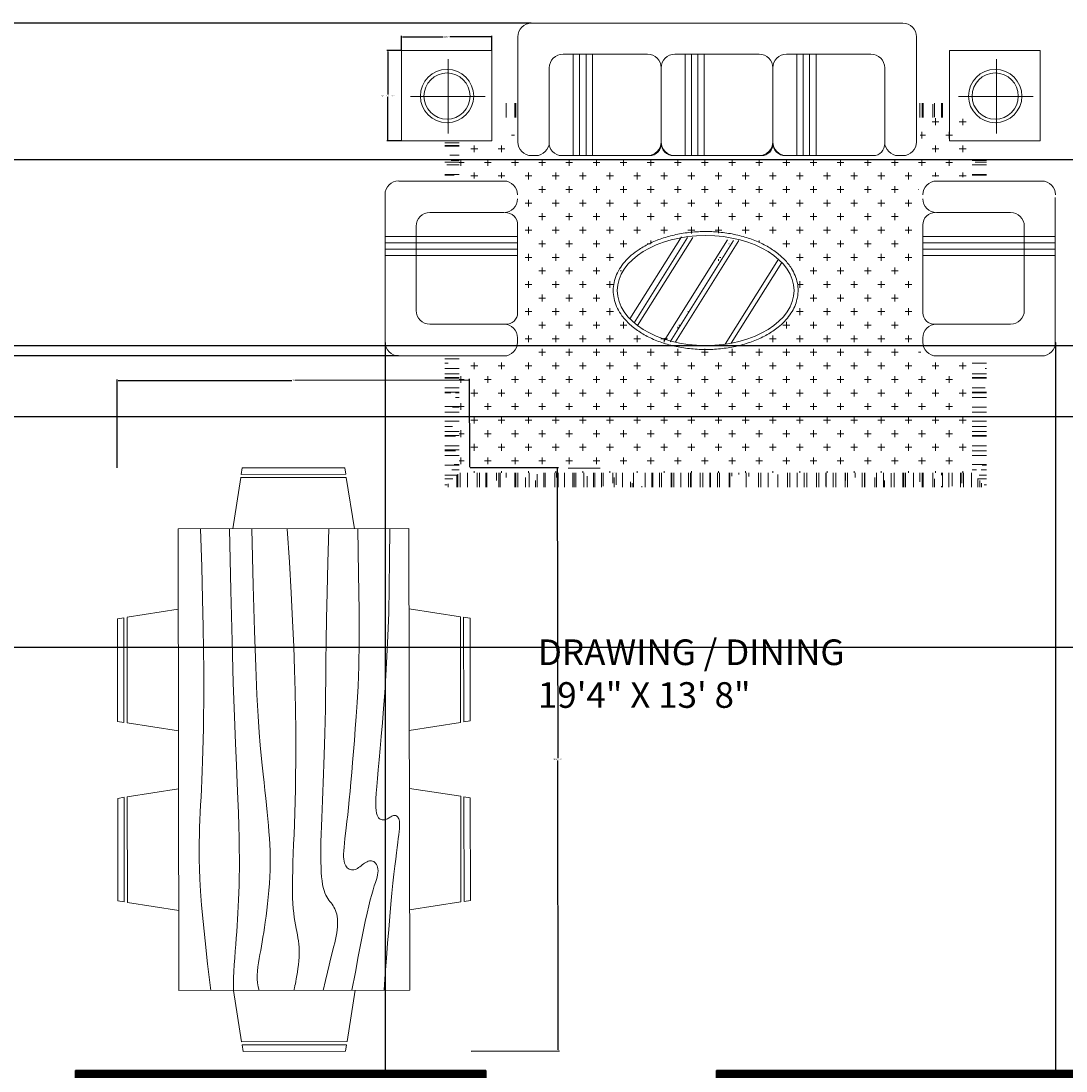
# Model space of a CAD drawing. Units: inches. Extents: x -24 to 516, y -23 to 640.
# Tile 3 of 5: x 139 to 302, y 288 to 452. Entities that reach past the tile are written whole.
import ezdxf

# ---------------------------------------------------------------- set-up
doc = ezdxf.new("R2010")
doc.units = ezdxf.units.IN
doc.header["$MEASUREMENT"] = 0
for name, color, linetype, lineweight in [('A-ANNO-DIMS', 2, 'Continuous', 18), ('A-AREA-IDEN', 7, 'Continuous', 18), ('A-FURN-PATT', 8, 'Continuous', 13), ('A-WALL', 7, 'Continuous', 35), ('furniture', 220, 'Continuous', 18)]:
    doc.layers.add(name, color=color, linetype=linetype, lineweight=lineweight)
doc.layers.add('A-WALL-PATT', color=198, linetype='Continuous', lineweight=13, true_color=0x2e0f2e)
doc.styles.get("Standard").update_dxf_attribs({"font": 'arial.ttf'})
doc.dimstyles.get("Standard").update_dxf_attribs({"dimtxt": 0.18, "dimasz": 0.18, "dimexe": 0.18, "dimexo": 0.0625, "dimgap": 0.09, "dimtad": 0, "dimtih": 1, "dimtoh": 1, "dimdec": 4, "dimzin": 0, "dimdsep": 46, "dimtxsty": 'Standard', "dimcen": 0.09, "dimadec": 0, "dimazin": 0, "dimtfac": 1, "dimtdec": 4, "dimtofl": 0, "dimtmove": 0, "dimatfit": 3, "dimfxl": 1, "dimtolj": 1, "dimtzin": 0, "dimarcsym": 0})

# ---------------------------------------------------------------- blocks, each defined once
blk = doc.blocks.new('Dining Set - 36 x 72 in.')
for p, q in [((-22, 27.5), (-22.1562, 26.50042)), ((-5.8416, 26.5), (-22.1534, 26.5)), ((-22, 27.5), (-6, 27.5)), ((-5.8437, 26.49966), (-6, 27.5)), ((6, 27.5), (5.8438, 26.50042)), ((22.1584, 26.5), (5.8466, 26.5)), ((6, 27.5), (22, 27.5)), ((22.1563, 26.49966), (22, 27.5)), ((-22.2343, 26.00059), (-23.4847, 17.99762)), ((-22.2304, 26), (-5.7608, 26)), ((-4.5152, 17.99762), (-5.7655, 25.99926)), ((5.7657, 26.00059), (4.5153, 17.99762)), ((5.7696, 26), (22.2392, 26)), ((23.4848, 17.99762), (22.2345, 25.99926)), ((36, 18), (-36, 18)), ((-36, 18), (-36, -18)), ((36, -18), (36, 18)), ((-44.0006, 8.23428), (-35.9976, 9.48474)), ((-44, 8.23041), (-44, -8.23915)), ((44.0006, 8.23428), (35.9976, 9.48474)), ((44, 8.23041), (44, -8.23915)), ((-45.5, 8), (-44.5004, 8.15617)), ((-45.5, 8), (-45.5, -8)), ((-44.5, -8.15843), (-44.5, 8.15338)), ((44.5, -8.15843), (44.5, 8.15338)), ((45.5, 8), (44.5005, 8.15617)), ((45.5, 8), (45.5, -8)), ((-44.4997, -8.15631), (-45.5, -8)), ((44.4997, -8.15631), (45.5, -8)), ((-35.9976, -9.48476), (-43.9993, -8.2345)), ((35.9976, -9.48476), (43.9993, -8.2345)), ((-36, -18), (36, -18)), ((-22.2343, -26.0006), (-23.4847, -17.99762)), ((-4.5152, -17.99762), (-5.7655, -25.99928)), ((5.7657, -26.0006), (4.5153, -17.99762)), ((23.4848, -17.99762), (22.2345, -25.99928)), ((-22.2304, -26), (-5.7608, -26)), ((5.7696, -26), (22.2392, -26)), ((-22, -27.5), (-22.1562, -26.50044)), ((-5.8416, -26.5), (-22.1534, -26.5)), ((-22, -27.5), (-6, -27.5)), ((-5.8437, -26.49967), (-6, -27.5)), ((6, -27.5), (5.8438, -26.50044)), ((22.1584, -26.5), (5.8466, -26.5)), ((6, -27.5), (22, -27.5)), ((22.1563, -26.49967), (22, -27.5))]:
    blk.add_line(p, q)
for points in [[(-36, 15), (-31.1772, 14.97754), (-26.8079, 14.91406), (-22.8538, 14.81543), (-19.276, 14.6875), (-16.0362, 14.53613), (-13.0957, 14.36718), (-10.4159, 14.18652), (-7.9583, 14), (-5.6904, 13.81315), (-3.6035, 13.63021), (-1.6954, 13.45508), (0.0365, 13.29166), (1.5945, 13.14388), (2.9811, 13.01562), (4.1988, 12.9108), (5.25, 12.83333), (6.1393, 12.78613), (6.8802, 12.76823), (7.4883, 12.77767), (7.9792, 12.8125), (8.3685, 12.87077), (8.6719, 12.95052), (8.9049, 13.0498), (9.0833, 13.16666), (9.2205, 13.29899), (9.3216, 13.44401), (9.3895, 13.59879), (9.4271, 13.76041), (9.4373, 13.92594), (9.4232, 14.09245), (9.3875, 14.257), (9.3333, 14.41666), (9.2638, 14.56917), (9.1836, 14.71484), (9.0975, 14.85465), (9.0104, 14.98958), (8.9272, 15.1206), (8.8529, 15.2487), (8.7922, 15.37483), (8.75, 15.5), (8.7305, 15.62467), (8.7344, 15.74739), (8.7617, 15.86621), (8.8125, 15.97916), (8.8867, 16.08431), (8.9844, 16.17968), (9.1055, 16.26334), (9.25, 16.33333), (9.4189, 16.38802), (9.6172, 16.42708), (9.8506, 16.45052), (10.125, 16.45833), (10.4463, 16.45052), (10.8203, 16.42708), (11.2529, 16.38802), (11.75, 16.33333), (12.3184, 16.26318), (12.9694, 16.17838), (13.7151, 16.07991), (14.5677, 15.96875), (15.5395, 15.84586), (16.6426, 15.71224), (17.8893, 15.56884), (19.2917, 15.41666), (20.859, 15.25667), (22.5879, 15.08984), (24.4721, 14.91715), (26.5052, 14.73958), (28.6809, 14.5581), (30.9929, 14.3737), (33.4347, 14.18733), (36, 14)], [(-36, 10), (-28.9766, 10.14274), (-23.1725, 10.20442), (-18.4241, 10.19775), (-14.5677, 10.13541), (-11.4399, 10.03011), (-8.877, 9.89453), (-6.7154, 9.74137), (-4.7917, 9.58333), (-2.9698, 9.43082), (-1.2246, 9.28515), (0.4415, 9.14534), (2.026, 9.01041), (3.5266, 8.87939), (4.9408, 8.7513), (6.266, 8.62516), (7.5, 8.5), (8.6411, 8.37549), (9.6914, 8.2539), (10.6538, 8.13818), (11.5312, 8.03125), (12.3267, 7.93603), (13.043, 7.85547), (13.6831, 7.79248), (14.25, 7.75), (14.7471, 7.7303), (15.1797, 7.73307), (15.5537, 7.75732), (15.875, 7.80208), (16.1494, 7.86637), (16.3828, 7.94922), (16.5811, 8.04964), (16.75, 8.16666), (16.8944, 8.29915), (17.0143, 8.44531), (17.1089, 8.60319), (17.1771, 8.77083), (17.218, 8.94629), (17.2305, 9.1276), (17.2137, 9.31282), (17.1667, 9.5), (17.0895, 9.6875), (16.987, 9.875), (16.8649, 10.0625), (16.7292, 10.25), (16.5856, 10.4375), (16.4401, 10.625), (16.2985, 10.8125), (16.1667, 11), (16.05, 11.18733), (15.9518, 11.3737), (15.8752, 11.5581), (15.8229, 11.73958), (15.798, 11.91715), (15.8034, 12.08984), (15.842, 12.25667), (15.9167, 12.41666), (16.0295, 12.56836), (16.1784, 12.70833), (16.3605, 12.83268), (16.5729, 12.9375), (16.8127, 13.01888), (17.0768, 13.07291), (17.3625, 13.0957), (17.6667, 13.08333), (17.9894, 13.03312), (18.3418, 12.94726), (18.7382, 12.82918), (19.1927, 12.68229), (19.7195, 12.51001), (20.3327, 12.31575), (21.0465, 12.10294), (21.875, 11.875), (22.8357, 11.63354), (23.959, 11.37304), (25.2786, 11.08618), (26.8282, 10.76562), (28.6414, 10.40405), (30.752, 9.99414), (33.1936, 9.52856), (36, 9)], [(-36, 5.5), (-30.7157, 5.3348), (-26.069, 5.20963), (-21.9946, 5.11767), (-18.4271, 5.05208), (-15.3009, 5.00602), (-12.5508, 4.97265), (-10.1112, 4.94515), (-7.9167, 4.91666), (-5.909, 4.88167), (-4.0586, 4.83984), (-2.3429, 4.79215), (-0.7396, 4.73958), (0.7739, 4.6831), (2.22, 4.6237), (3.6213, 4.56233), (5, 4.5), (6.373, 4.43782), (7.7344, 4.3776), (9.0723, 4.32129), (10.375, 4.27083), (11.6309, 4.22819), (12.8281, 4.19531), (13.9551, 4.17415), (15, 4.16666), (15.954, 4.17448), (16.819, 4.19791), (17.6001, 4.23698), (18.3021, 4.29166), (18.9299, 4.36198), (19.4883, 4.44791), (19.9823, 4.54948), (20.4167, 4.66666), (20.7969, 4.79899), (21.1302, 4.94401), (21.4245, 5.09879), (21.6875, 5.26041), (21.9271, 5.42594), (22.1511, 5.59245), (22.3672, 5.757), (22.5834, 5.91666), (22.8065, 6.06868), (23.0404, 6.21093), (23.2879, 6.34147), (23.5521, 6.45833), (23.8358, 6.55957), (24.142, 6.64323), (24.4735, 6.70735), (24.8334, 6.75), (25.2235, 6.76969), (25.642, 6.76692), (26.0858, 6.74267), (26.5521, 6.69791), (27.0379, 6.63362), (27.5404, 6.55078), (28.0565, 6.45036), (28.5834, 6.33333), (29.1242, 6.19987), (29.7071, 6.04687), (30.3661, 5.87044), (31.1354, 5.66666), (32.0493, 5.43164), (33.142, 5.16146), (34.4475, 4.85221), (36, 4.5)], [(-36, -1), (-30.7915, -0.6591), (-26.0195, -0.38216), (-21.6519, -0.16284), (-17.6563, 0.00521), (-14.0005, 0.12833), (-10.6523, 0.21289), (-7.5796, 0.26522), (-4.75, 0.29166), (-2.134, 0.29793), (0.2878, 0.28711), (2.5317, 0.26163), (4.6146, 0.22396), (6.5529, 0.17651), (8.3633, 0.12174), (10.0623, 0.06209), (11.6667, 0), (13.1899, -0.06201), (14.6341, -0.1211), (15.9982, -0.17432), (17.2813, -0.21875), (18.4823, -0.25147), (19.6003, -0.26953), (20.6343, -0.27002), (21.5834, -0.25), (22.4481, -0.20768), (23.2357, -0.14584), (23.9549, -0.06836), (24.6146, 0.02083), (25.2235, 0.11784), (25.7904, 0.21875), (26.3241, 0.31966), (26.8334, 0.41666), (27.3265, 0.50618), (27.8099, 0.58593), (28.2894, 0.65397), (28.7709, 0.70833), (29.2601, 0.74707), (29.763, 0.76823), (30.2855, 0.76985), (30.8334, 0.75), (31.4088, 0.70784), (31.9994, 0.64713), (32.589, 0.57275), (33.1615, 0.48958), (33.7008, 0.4025), (34.1908, 0.3164), (34.6153, 0.23616), (34.9584, 0.16666), (35.2099, 0.11165), (35.3848, 0.07031), (35.504, 0.04069), (35.5886, 0.02083), (35.6594, 0.00879), (35.7377, 0.0026), (35.8442, 0.00032), (36, 0)], [(-36, -6.5), (-27.1843, -6.31267), (-20.084, -6.1263), (-14.469, -5.9419), (-10.1094, -5.76042), (-6.7752, -5.58285), (-4.2363, -5.41016), (-2.2629, -5.24333), (-0.625, -5.08334), (0.8708, -4.93099), (2.2715, -4.78646), (3.5872, -4.64974), (4.8281, -4.52084), (6.0046, -4.39974), (7.127, -4.28646), (8.2053, -4.18099), (9.25, -4.08334), (10.2705, -3.99382), (11.2734, -3.91407), (12.2647, -3.84603), (13.25, -3.79167), (14.2354, -3.75293), (15.2266, -3.73177), (16.2295, -3.73015), (17.25, -3.75), (18.2912, -3.79248), (19.3451, -3.85547), (20.4009, -3.93604), (21.4479, -4.03125), (22.4754, -4.13819), (23.4727, -4.25391), (24.4289, -4.37549), (25.3334, -4.5), (26.1785, -4.62492), (26.9694, -4.74935), (27.7145, -4.87281), (28.4219, -4.99479), (29.1, -5.11483), (29.7572, -5.23242), (30.4016, -5.34709), (31.0417, -5.45834), (31.6837, -5.56437), (32.3262, -5.65821), (32.9658, -5.73153), (33.599, -5.77604), (34.2224, -5.78345), (34.8327, -5.74545), (35.4264, -5.65373), (36, -5.5)], [(-36, -10), (-26.4022, -9.81299), (-18.4675, -9.62891), (-11.9839, -9.45069), (-6.7396, -9.28125), (-2.5226, -9.12354), (0.8789, -8.98047), (3.6769, -8.85498), (6.0833, -8.75), (8.2767, -8.66765), (10.3021, -8.60677), (12.1712, -8.56543), (13.8958, -8.54167), (15.4876, -8.53353), (16.9583, -8.53907), (18.3197, -8.55632), (19.5834, -8.58334), (20.7616, -8.61841), (21.8685, -8.66081), (22.9188, -8.71004), (23.9271, -8.76563), (24.9081, -8.82707), (25.8763, -8.89388), (26.8465, -8.96558), (27.8334, -9.04167), (28.8474, -9.12118), (29.8828, -9.20117), (30.93, -9.27824), (31.9792, -9.34896), (33.0205, -9.40991), (34.0443, -9.45768), (35.0407, -9.48885), (36, -9.5)], [(-36, -14.5), (-30.0881, -14.33513), (-25.0332, -14.21224), (-20.7312, -14.12647), (-17.0781, -14.07292), (-13.97, -14.04671), (-11.3027, -14.04297), (-8.9724, -14.05681), (-6.875, -14.08334), (-4.9224, -14.11833), (-3.0905, -14.16016), (-1.3709, -14.20785), (0.2448, -14.26042), (1.7647, -14.3169), (3.1973, -14.3763), (4.5507, -14.43767), (5.8333, -14.5), (7.0554, -14.5621), (8.235, -14.62175), (9.3922, -14.67652), (10.5469, -14.72396), (11.7192, -14.76164), (12.929, -14.78711), (14.1965, -14.79794), (15.5417, -14.79167), (16.9933, -14.76424), (18.6152, -14.70508), (20.4804, -14.60197), (22.6615, -14.44271), (25.2312, -14.21509), (28.2624, -13.9069), (31.8277, -13.50594), (36, -13)]]:
    blk.add_lwpolyline(points)
blk = doc.blocks.new('END-TABLE-WITH-LAMP')
for p, q in [((14.11, 14.11), (0, 14.11)), ((0, 14.11), (0, 0)), ((14.11, 0), (14.11, 14.11)), ((7.3, 1.14), (7.3, 12.78)), ((1.4, 6.95), (13.04, 6.95)), ((0, 0), (14.11, 0))]:
    blk.add_line(p, q)
for radius in [4.16, 3.6]:
    blk.add_circle((7.11, 7), radius)
blk = doc.blocks.new('*D25')
at = {"layer": 'A-ANNO-DIMS', "color": 0, "lineweight": -2, "transparency": 16777216}
for p, q in [((197.87, 447.09), (195.63, 447.09)), ((195.81, 446.91), (195.81, 440.21)), ((195.81, 433.16), (195.81, 439.85)), ((197.87, 432.98), (195.63, 432.98))]:
    blk.add_line(p, q, dxfattribs=at)
at = {"layer": 'A-ANNO-DIMS', "color": 0, "transparency": 16777216}
for points in [[(195.78, 446.91), (195.84, 446.91), (195.81, 447.09)], [(195.78, 433.16), (195.84, 433.16), (195.81, 432.98)]]:
    blk.add_solid(points, dxfattribs=at)
at = {"layer": 'Defpoints', "color": 0, "transparency": 16777216}
for p in [(195.81, 447.09), (197.93, 447.09), (197.93, 432.98)]:
    blk.add_point(p, dxfattribs=at)
at = {"layer": 'A-ANNO-DIMS', "color": 0, "transparency": 16777216, "insert": (195.81, 440.03), "char_height": 0.18, "attachment_point": 5}
blk.add_mtext('\\A1;LAMP TABLE 14 TYP.', dxfattribs=at)
blk = doc.blocks.new('*D26')
at = {"layer": 'A-ANNO-DIMS', "color": 0, "lineweight": -2, "transparency": 16777216}
for p, q in [((197.93, 447.15), (197.93, 449.38)), ((198.11, 449.2), (204.46, 449.2)), ((211.86, 449.2), (205.5, 449.2)), ((212.04, 447.15), (212.04, 449.38))]:
    blk.add_line(p, q, dxfattribs=at)
at = {"layer": 'A-ANNO-DIMS', "color": 0, "transparency": 16777216}
for points in [[(198.11, 449.23), (198.11, 449.17), (197.93, 449.2)], [(211.86, 449.23), (211.86, 449.17), (212.04, 449.2)]]:
    blk.add_solid(points, dxfattribs=at)
at = {"layer": 'Defpoints', "color": 0, "transparency": 16777216}
for p in [(212.04, 449.2), (197.93, 447.09), (212.04, 447.09)]:
    blk.add_point(p, dxfattribs=at)
at = {"layer": 'A-ANNO-DIMS', "color": 0, "transparency": 16777216, "insert": (204.98, 449.2), "char_height": 0.18, "attachment_point": 5}
blk.add_mtext('\\A1;14 TYP.', dxfattribs=at)
blk = doc.blocks.new('*D31')
at = {"layer": 'A-ANNO-DIMS', "color": 0, "lineweight": -2, "transparency": 16777216}
for p, q in [((208.65, 382.03), (222.42, 382.05)), ((222.24, 381.87), (222.31, 336.73)), ((222.38, 291.23), (222.31, 336.37)), ((208.79, 291.03), (222.56, 291.05))]:
    blk.add_line(p, q, dxfattribs=at)
at = {"layer": 'A-ANNO-DIMS', "color": 0, "transparency": 16777216}
for points in [[(222.27, 381.87), (222.21, 381.87), (222.24, 382.05)], [(222.41, 291.23), (222.35, 291.23), (222.38, 291.05)]]:
    blk.add_solid(points, dxfattribs=at)
at = {"layer": 'Defpoints', "color": 0, "transparency": 16777216}
for p in [(208.59, 382.03), (208.73, 291.03), (222.38, 291.05)]:
    blk.add_point(p, dxfattribs=at)
at = {"layer": 'A-ANNO-DIMS', "color": 0, "transparency": 16777216, "insert": (222.31, 336.55), "char_height": 0.18, "attachment_point": 5}
blk.add_mtext('\\A1;DINING SET 91', dxfattribs=at)
blk = doc.blocks.new('*D32')
at = {"layer": 'A-ANNO-DIMS', "color": 0, "lineweight": -2, "transparency": 16777216}
for p, q in [((153.59, 382), (153.57, 395.77)), ((153.75, 395.59), (180.85, 395.63)), ((208.39, 395.68), (181.29, 395.64)), ((208.59, 382.09), (208.57, 395.86))]:
    blk.add_line(p, q, dxfattribs=at)
at = {"layer": 'A-ANNO-DIMS', "color": 0, "transparency": 16777216}
for points in [[(153.75, 395.62), (153.75, 395.56), (153.57, 395.59)], [(208.39, 395.71), (208.39, 395.65), (208.57, 395.68)]]:
    blk.add_solid(points, dxfattribs=at)
at = {"layer": 'Defpoints', "color": 0, "transparency": 16777216}
for p in [(208.57, 395.68), (153.59, 381.94), (208.59, 382.03)]:
    blk.add_point(p, dxfattribs=at)
at = {"layer": 'A-ANNO-DIMS', "color": 0, "transparency": 16777216, "insert": (181.07, 395.63), "char_height": 0.18, "attachment_point": 5}
blk.add_mtext('\\A1;55', dxfattribs=at)
blk = doc.blocks.new('*D48')
at = {"layer": 'A-ANNO-DIMS', "color": 0, "lineweight": -2, "transparency": 16777216}
for p, q in [((99.15, 390.01), (516.45, 390.01)), ((516.27, 389.83), (516.27, 372.2)), ((516.27, 354.19), (516.27, 371.83)), ((99.15, 354.01), (516.45, 354.01))]:
    blk.add_line(p, q, dxfattribs=at)
at = {"layer": 'A-ANNO-DIMS', "color": 0, "transparency": 16777216}
for points in [[(516.24, 389.83), (516.3, 389.83), (516.27, 390.01)], [(516.24, 354.19), (516.3, 354.19), (516.27, 354.01)]]:
    blk.add_solid(points, dxfattribs=at)
at = {"layer": 'Defpoints', "color": 0, "transparency": 16777216}
for p in [(99.09, 390.01), (516.27, 390.01), (99.09, 354.01)]:
    blk.add_point(p, dxfattribs=at)
at = {"layer": 'A-ANNO-DIMS', "color": 0, "transparency": 16777216, "insert": (516.27, 372.01), "char_height": 0.18, "attachment_point": 5}
blk.add_mtext('\\A1;36', dxfattribs=at)
blk = doc.blocks.new('*D52')
at = {"layer": 'A-ANNO-DIMS', "color": 0, "lineweight": -2, "transparency": 16777216}
for p, q in [((392.03, 430.01), (-24.28, 430.01)), ((-24.1, 429.83), (-24.1, 415.7)), ((-24.1, 401.19), (-24.1, 415.33)), ((392.03, 401.01), (-24.28, 401.01))]:
    blk.add_line(p, q, dxfattribs=at)
at = {"layer": 'A-ANNO-DIMS', "color": 0, "transparency": 16777216}
for points in [[(-24.13, 429.83), (-24.07, 429.83), (-24.1, 430.01)], [(-24.13, 401.19), (-24.07, 401.19), (-24.1, 401.01)]]:
    blk.add_solid(points, dxfattribs=at)
at = {"layer": 'Defpoints', "color": 0, "transparency": 16777216}
for p in [(-24.1, 430.01), (392.09, 430.01), (392.09, 401.01)]:
    blk.add_point(p, dxfattribs=at)
at = {"layer": 'A-ANNO-DIMS', "color": 0, "transparency": 16777216, "insert": (-24.1, 415.51), "char_height": 0.18, "attachment_point": 5}
blk.add_mtext('\\A1;29', dxfattribs=at)
blk = doc.blocks.new('*D55')
at = {"layer": 'A-ANNO-DIMS', "color": 0, "lineweight": -2, "transparency": 16777216}
for p, q in [((195.37, 401.52), (195.37, -23.35)), ((299.94, 401.52), (299.94, -23.35)), ((195.55, -23.17), (247.2, -23.17)), ((299.76, -23.17), (248.11, -23.17))]:
    blk.add_line(p, q, dxfattribs=at)
at = {"layer": 'A-ANNO-DIMS', "color": 0, "transparency": 16777216}
for points in [[(195.55, -23.14), (195.55, -23.2), (195.37, -23.17)], [(299.76, -23.14), (299.76, -23.2), (299.94, -23.17)]]:
    blk.add_solid(points, dxfattribs=at)
at = {"layer": 'Defpoints', "color": 0, "transparency": 16777216}
for p in [(195.37, 401.58), (299.94, 401.58), (299.94, -23.17)]:
    blk.add_point(p, dxfattribs=at)
at = {"layer": 'A-ANNO-DIMS', "color": 0, "transparency": 16777216, "insert": (247.66, -23.17), "char_height": 0.18, "attachment_point": 5}
blk.add_mtext('\\A1;104.57', dxfattribs=at)
blk = doc.blocks.new('*D56')
at = {"layer": 'A-ANNO-DIMS', "color": 0, "lineweight": -2, "transparency": 16777216}
for p, q in [((218.16, 451.37), (-24.28, 451.37)), ((-24.1, 451.19), (-24.1, 425.59)), ((-24.1, 399.62), (-24.1, 425.22)), ((197.45, 399.44), (-24.28, 399.44))]:
    blk.add_line(p, q, dxfattribs=at)
at = {"layer": 'A-ANNO-DIMS', "color": 0, "transparency": 16777216}
for points in [[(-24.13, 451.19), (-24.07, 451.19), (-24.1, 451.37)], [(-24.13, 399.62), (-24.07, 399.62), (-24.1, 399.44)]]:
    blk.add_solid(points, dxfattribs=at)
at = {"layer": 'Defpoints', "color": 0, "transparency": 16777216}
for p in [(218.23, 451.37), (-24.1, 399.44), (197.51, 399.44)]:
    blk.add_point(p, dxfattribs=at)
at = {"layer": 'A-ANNO-DIMS', "color": 0, "transparency": 16777216, "insert": (-24.1, 425.4), "char_height": 0.18, "attachment_point": 5}
blk.add_mtext('\\A1;51.92', dxfattribs=at)

msp = doc.modelspace()

# ---------------------------------------------------------------- hatches: boundary and pattern name
at = {"layer": 'A-FURN-PATT'}
h = msp.add_hatch(dxfattribs=at)
h.set_pattern_fill('AR-RROOF', color=256, scale=2.507942, angle=540, style=0)
h.set_pattern_definition([(90, (563.2087, 188.401), (2.257148, 4.965726), [33.85722, -4.5143, 11.28574, -2.25715]), (90, (564.3373, 191.403), (3.002007, -2.257148), [6.771445, -0.74486, 13.54289, -1.69286]), (90, (565.1273, 189.5296), (1.5122893, 11.7371705), [18.057185, -3.16001, 9.028593, -2.25715])])
h.paths.add_polyline_path([(214.107, 438.879), (216.089, 438.879), (216.089, 436.622), (214.107, 436.622)])
h.paths.add_polyline_path([(206.938, 381.239), (286.936, 381.239), (289.193, 378.982), (204.681, 378.982)])
h.paths.add_polyline_path([(278.262, 438.879), (283.498, 438.879), (283.202, 436.622), (278.262, 436.622)])
h = msp.add_hatch(dxfattribs=at)
h.set_pattern_fill('CROSS', color=256, scale=9.404784, angle=450, style=0)
h.set_pattern_definition([(180, (563.2087, 188.401), (-2.116076, 2.116076), [1.058038, -3.174115]), (90, (562.6797, 187.872), (2.116076, 2.116076), [1.058038, -3.174115])])
h.paths.add_polyline_path([(206.938, 398.747), (214.85, 398.975), (216.478, 399.111), (216.614, 425.549), (215.664, 427.176), (206.938, 427.082), (206.938, 432.98), (214.107, 432.98), (214.107, 436.622), (215.497, 436.622), (215.664, 430.294), (277.39, 430.023), (278.882, 430.972), (278.803, 436.622), (284.171, 436.622), (286.936, 436.222), (286.936, 427.298), (280.374, 427.447), (278.611, 425.549), (278.204, 402.771), (279.153, 399.111), (286.936, 398.86), (286.936, 381.239), (206.938, 381.239)])
h.paths.add_polyline_path([(243.475, 401.28), (253.513, 401.415), (259.076, 406.025), (259.89, 408.059), (259.89, 410.635), (259.483, 412.533), (258.262, 415.109), (255.684, 416.194), (252.699, 417.685), (249.444, 418.363), (245.509, 418.77), (237.234, 417.279), (232.486, 413.889), (231.536, 408.466), (233.029, 405.347), (236.963, 402.636)], flags=16)
edge = h.paths.add_edge_path(flags=0)
edge.add_line((240.138, 402.488), (249.041, 417.293))
edge.add_ellipse((245.565, 394.403), major_axis=(16.371, 16.371), ratio=1, start_angle=35.87674, end_angle=36.36513, ccw=False)
edge.add_line((249.236, 417.262), (240.325, 402.443))
edge.add_ellipse((245.565, 424.995), major_axis=(16.371, -16.371), ratio=1, start_angle=301.44538, end_angle=301.92024, ccw=False)
edge.add_line((240.138, 402.488), (240.138, 402.488))
edge.add_ellipse((243.745, 417.44), major_axis=(10.876, -10.876), ratio=0.9999999, start_angle=301.43989, end_angle=301.45625)
edge.add_line((240.142, 402.487), (240.142, 402.487))
edge.add_line((240.142, 402.487), (240.142, 402.487))
edge.add_line((240.142, 402.487), (240.142, 402.487))
edge.add_line((240.142, 402.487), (240.142, 402.487))
edge.add_line((240.142, 402.487), (240.142, 402.487))
edge.add_ellipse((243.745, 417.44), major_axis=(10.876, 10.876), ratio=1, start_angle=211.43989, end_angle=211.45624, ccw=False)
h = msp.add_hatch(dxfattribs=at)
h.set_pattern_fill('AR-RROOF', color=256, scale=2.507942, angle=450, style=0)
h.set_pattern_definition([(180, (563.2087, 188.401), (-4.965726, 2.257148), [33.85722, -4.5143, 11.28574, -2.25715]), (180, (560.2067, 189.5296), (2.257148, 3.002007), [6.771445, -0.74486, 13.54289, -1.69286]), (180, (562.0801, 190.3196), (-11.7371705, 1.5122893), [18.057185, -3.16001, 9.028593, -2.25715])])
h.paths.add_polyline_path([(204.681, 432.98), (206.938, 432.98), (206.938, 426.729), (204.681, 426.729)])
h.paths.add_polyline_path([(204.681, 399.442), (206.938, 399.442), (206.938, 381.239), (204.681, 378.982)])
h.paths.add_polyline_path([(286.936, 399.442), (289.193, 399.442), (289.193, 378.982), (286.936, 381.239)])
h.paths.add_polyline_path([(286.936, 430.245), (289.193, 429.948), (289.193, 426.729), (286.936, 426.729)])
at = {"layer": 'A-WALL-PATT'}
h = msp.add_hatch(dxfattribs=at)
h.set_pattern_fill('ANSI31', color=256)
h.set_pattern_definition([(45, (-12045.43418, -42625.98622), (-0.08838834765, 0.08838834765), [])])
h.paths.add_polyline_path([(161.63, 139.013), (155.088, 139.013), (155.088, 283.013), (203.088, 283.013), (203.088, 171.013), (208.088, 171.013), (208.088, 283.013), (211.088, 283.013), (211.088, 288.013), (208.088, 288.013), (147.088, 288.013), (147.088, 283.013), (150.088, 283.013), (150.088, 139.013), (87.664, 139.013), (87.664, 134.513), (87.664, 130.013), (161.63, 130.013)])
h.paths.add_polyline_path([(256.352, 139.013), (208.088, 139.013), (208.088, 142.013), (203.088, 142.013), (203.088, 139.013), (185.63, 139.013), (185.63, 130.013), (256.352, 130.013)])
h.paths.add_polyline_path([(345.088, 326.013), (336.088, 326.013), (336.088, 288.013), (247.088, 288.013), (247.088, 283.013), (340.088, 283.013), (340.088, 139.013), (292.352, 139.013), (292.352, 134.513), (292.352, 130.013), (345.088, 130.013)])
h.paths.add_polyline_path([(51.664, 139.013), (15.088, 139.013), (15.088, 195.946), (10.588, 195.946), (6.088, 195.946), (6.088, 130.013), (51.664, 130.013)])
h.paths.add_polyline_path([(15.088, 283.013), (111.088, 283.013), (111.088, 288.013), (104.088, 288.013), (104.088, 354.013), (99.088, 354.013), (99.088, 288.013), (15.088, 288.013), (15.088, 324.046), (10.588, 324.046), (6.088, 324.046), (6.088, 231.946), (15.088, 231.946)])
h.paths.add_polyline_path([(15.088, 398.013), (99.088, 398.013), (99.088, 390.013), (104.088, 390.013), (104.088, 393.013), (104.088, 407.013), (99.088, 407.013), (99.088, 404.013), (15.088, 404.013), (15.088, 416.474), (10.588, 416.474), (6.088, 416.474), (6.088, 360.046), (15.088, 360.046)])
h.paths.add_polyline_path([(15.088, 518.753), (10.588, 518.753), (6.088, 518.753), (6.088, 440.474), (15.088, 440.474), (15.088, 452.013), (99.088, 452.013), (99.088, 436.013), (104.088, 436.013), (104.088, 452.013), (111.088, 452.013), (111.088, 457.013), (15.088, 457.013)])

# ---------------------------------------------------------------- linework, layer by layer
at = {"layer": 'A-WALL'}
for p, q in [((147.088, 288.013), (155.088, 288.013)), ((211.088, 288.013), (147.088, 288.013)), ((150.088, 288.013), (147.088, 288.013)), ((147.088, 288.013), (147.088, 283.013)), ((208.088, 288.013), (211.088, 288.013)), ((211.088, 288.013), (211.088, 283.013)), ((336.088, 288.013), (247.088, 288.013)), ((247.088, 283.013), (247.088, 288.013))]:
    msp.add_line(p, q, dxfattribs=at)
at = {"layer": 'furniture'}
for p, q in [((276.125, 451.366), (218.226, 451.366)), ((216.089, 449.229), (216.089, 432.824)), ((278.262, 432.824), (278.262, 449.229)), ((223.132, 446.512), (236.293, 446.512)), ((224.734, 430.736), (224.734, 446.512)), ((225.73, 430.736), (225.73, 446.512)), ((226.725, 430.736), (226.725, 446.512)), ((227.721, 430.736), (227.721, 446.512)), ((240.573, 446.512), (253.735, 446.512)), ((242.176, 430.736), (242.176, 446.512)), ((243.171, 430.736), (243.171, 446.512)), ((244.167, 430.736), (244.167, 446.512)), ((245.162, 430.736), (245.162, 446.512)), ((258.009, 446.512), (271.171, 446.512)), ((259.612, 430.736), (259.612, 446.512)), ((260.607, 430.736), (260.607, 446.512)), ((261.603, 430.736), (261.603, 446.512)), ((262.598, 430.736), (262.598, 446.512)), ((220.995, 432.824), (220.995, 444.375)), ((238.43, 444.375), (238.43, 432.824)), ((255.872, 432.824), (255.872, 444.375)), ((273.308, 444.375), (273.308, 432.824)), ((218.226, 430.687), (218.858, 430.687)), ((222.937, 430.687), (236.633, 430.687)), ((240.379, 430.687), (254.075, 430.687)), ((257.815, 430.687), (271.511, 430.687)), ((275.445, 430.687), (276.228, 430.687)), ((197.509, 426.729), (213.915, 426.729)), ((297.804, 426.729), (281.398, 426.729)), ((195.372, 424.64), (195.372, 401.619)), ((299.881, 401.16), (299.881, 424.181)), ((213.915, 421.823), (202.364, 421.823)), ((281.398, 421.823), (292.949, 421.823)), ((200.227, 406.525), (200.227, 419.686)), ((216.052, 419.881), (216.052, 406.185)), ((279.261, 419.881), (279.261, 406.185)), ((295.086, 419.686), (295.086, 406.525)), ((216.003, 418.084), (195.372, 418.084)), ((241.617, 418.036), (233.579, 405.22)), ((242.56, 417.918), (234.218, 404.619)), ((243.384, 417.918), (234.767, 404.179)), ((279.31, 418.084), (299.94, 418.084)), ((216.003, 417.088), (195.372, 417.088)), ((216.003, 416.093), (195.372, 416.093)), ((248.803, 417.565), (238.908, 401.788)), ((249.746, 417.447), (239.85, 401.671)), ((250.57, 417.447), (240.675, 401.671)), ((279.31, 417.088), (299.94, 417.088)), ((279.31, 416.093), (299.94, 416.093)), ((216.003, 415.097), (195.372, 415.097)), ((256.726, 414.529), (248.42, 401.287)), ((279.31, 415.097), (299.94, 415.097)), ((257.239, 414.032), (249.339, 401.437)), ((214.11, 404.382), (202.364, 404.388)), ((281.203, 404.382), (292.949, 404.388)), ((216.052, 402.259), (216.052, 401.579)), ((279.261, 402.259), (279.261, 401.579)), ((213.915, 399.442), (197.509, 399.442)), ((281.398, 399.442), (297.804, 399.442)), ((223.934, 381.938), (228.934, 381.938))]:
    msp.add_line(p, q, dxfattribs=at)
for centre, radius, start, end in [((218.226, 449.229), 2.137, 90, 180), ((276.125, 449.229), 2.137, 0, 90), ((223.132, 444.375), 2.137, 90, 180), ((236.293, 444.375), 2.137, 0, 90), ((240.573, 444.375), 2.137, 90, 180), ((253.735, 444.375), 2.137, 0, 90), ((258.009, 444.375), 2.137, 90, 180), ((271.171, 444.375), 2.137, 0, 90), ((218.226, 432.824), 2.137, 180, 270), ((218.858, 432.824), 2.137, 270, 0), ((222.922, 432.625), 1.938, 174.10185, 270.44553), ((236.299, 432.824), 2.137, 270, 0), ((236.633, 432.486), 1.799, 270, 2.98595), ((240.567, 432.824), 2.137, 180, 270), ((240.357, 432.608), 1.921, 179.37008, 270.65888), ((253.735, 432.824), 2.137, 270, 0), ((254.075, 432.486), 1.799, 270, 2.98595), ((258.009, 432.824), 2.137, 180, 270), ((257.793, 432.608), 1.921, 179.37008, 270.65888), ((271.511, 432.486), 1.799, 270, 2.98595), ((275.445, 432.824), 2.137, 180, 270), ((276.125, 432.824), 2.137, 270, 0), ((197.509, 424.631), 2.137, 90, 180), ((213.915, 424.592), 2.137, 0, 90), ((281.398, 424.592), 2.137, 90, 180), ((297.804, 424.592), 2.137, 0, 90), ((213.915, 423.96), 2.137, 270, 0), ((281.398, 423.96), 2.137, 180, 270), ((202.364, 419.686), 2.137, 90, 180), ((214.131, 419.903), 1.921, 359.34112, 90.62992), ((281.182, 419.903), 1.921, 89.37008, 180.65888), ((292.949, 419.686), 2.137, 0, 90), ((202.364, 406.525), 2.137, 180, 270), ((214.252, 406.185), 1.799, 267.01405, 0), ((281.061, 406.185), 1.799, 180, 272.98595), ((292.949, 406.525), 2.137, 270, 0), ((213.915, 402.259), 2.137, 0, 90), ((281.398, 402.259), 2.137, 90, 180), ((197.509, 401.579), 2.137, 180, 270), ((213.915, 401.579), 2.137, 270, 0), ((281.398, 401.579), 2.137, 180, 270), ((297.804, 401.579), 2.137, 270, 0)]:
    msp.add_arc(centre, radius, start, end, dxfattribs=at)
at = {"layer": 'furniture', "extrusion": (0, 0, -1)}
msp.add_ellipse((245.384, 409.652), major_axis=(13.789, 0), ratio=0.6218602, start_param=4.712389, end_param=10.9955743, dxfattribs=at)
at = {"layer": 'furniture'}
msp.add_open_spline([(259.8, 409.652), (259.8, 409.379), (259.781, 409.106), (259.707, 408.564), (259.651, 408.295), (259.471, 407.646), (259.329, 407.271), (258.973, 406.538), (258.761, 406.18), (258.271, 405.488), (257.994, 405.154), (257.38, 404.513), (257.044, 404.206), (256.171, 403.504), (255.608, 403.124), (254.392, 402.433), (253.74, 402.122), (252.364, 401.574), (251.64, 401.337), (250.142, 400.945), (249.367, 400.79), (247.788, 400.563), (246.984, 400.491), (245.368, 400.435), (244.556, 400.45), (242.947, 400.566), (242.151, 400.667), (240.595, 400.952), (239.835, 401.136), (238.375, 401.584), (237.674, 401.847), (236.35, 402.446), (235.726, 402.782), (234.575, 403.52), (234.047, 403.921), (233.103, 404.781), (232.686, 405.239), (232.061, 406.091), (231.827, 406.475), (231.439, 407.264), (231.286, 407.67), (231.065, 408.494), (230.998, 408.912), (230.953, 409.752), (230.975, 410.173), (231.107, 411.008), (231.218, 411.421), (231.522, 412.23), (231.716, 412.625), (232.182, 413.392), (232.454, 413.763), (233.069, 414.475), (233.412, 414.816), (234.162, 415.464), (234.57, 415.77), (235.562, 416.425), (236.164, 416.76), (237.446, 417.362), (238.125, 417.629), (239.542, 418.086), (240.279, 418.278), (241.793, 418.581), (242.569, 418.692), (244.14, 418.834), (244.934, 418.863), (246.52, 418.839), (247.311, 418.786), (248.87, 418.597), (249.637, 418.462), (251.127, 418.114), (251.849, 417.9), (253.231, 417.4), (253.889, 417.113), (255.125, 416.471), (255.703, 416.117), (256.76, 415.348), (257.24, 414.934), (258.088, 414.054), (258.456, 413.588), (258.989, 412.738), (259.182, 412.363), (259.492, 411.596), (259.61, 411.205), (259.762, 410.426), (259.8, 410.039), (259.8, 409.652)], degree=3, knots=[3.1415927, 3.1415927, 3.1415927, 3.1415927, 3.2269172, 3.2269172, 3.3122416, 3.3122416, 3.4342667, 3.4342667, 3.5562918, 3.5562918, 3.6783168, 3.6783168, 3.8003419, 3.8003419, 3.9715738, 3.9715738, 4.1428058, 4.1428058, 4.3140377, 4.3140377, 4.4852697, 4.4852697, 4.6565016, 4.6565016, 4.8277335, 4.8277335, 4.9989655, 4.9989655, 5.1701974, 5.1701974, 5.3414293, 5.3414293, 5.5126613, 5.5126613, 5.6838932, 5.6838932, 5.8551252, 5.8551252, 5.9866911, 5.9866911, 6.118257, 6.118257, 6.2498229, 6.2498229, 6.3813888, 6.3813888, 6.5129547, 6.5129547, 6.6445207, 6.6445207, 6.7760866, 6.7760866, 6.9076525, 6.9076525, 7.0392184, 7.0392184, 7.2070156, 7.2070156, 7.3748129, 7.3748129, 7.5426101, 7.5426101, 7.7104073, 7.7104073, 7.8782046, 7.8782046, 8.0460018, 8.0460018, 8.213799, 8.213799, 8.3815962, 8.3815962, 8.5493935, 8.5493935, 8.7171907, 8.7171907, 8.8849879, 8.8849879, 9.0527852, 9.0527852, 9.178207, 9.178207, 9.3036288, 9.3036288, 9.424778, 9.424778, 9.424778, 9.424778], dxfattribs=at)

# ---------------------------------------------------------------- block references
for p in [(197.93, 432.98), (283.437, 432.98)]:
    msp.add_blockref('END-TABLE-WITH-LAMP', p, dxfattribs=at)
at = {"layer": 'furniture', "rotation": 270.0891389700014}
msp.add_blockref('Dining Set - 36 x 72 in.', (181.162, 336.485), dxfattribs=at)

# ---------------------------------------------------------------- texts
at = {"layer": 'A-AREA-IDEN', "insert": (217.993, 355.228), "char_height": 4, "attachment_point": 1}
msp.add_mtext_dynamic_manual_height_columns(' DRAWING / DINING\\P 19\'4" X 13\' 8"', width=73.41269, gutter_width=1, heights=[0], dxfattribs=at)

# ---------------------------------------------------------------- dimensions: what is measured, and where the dimension line sits
at = {"layer": 'A-ANNO-DIMS'}
for base, p1, p2, angle, override, picture, middle in [((-24.097, 399.442), (218.226, 451.366), (197.509, 399.442), 90, {"dimdec": 2, "dimlfac": 1, "dimrnd": 0, "dimzin": 0, "dimdsep": 46, "dimlunit": 2}, '*D56', (-24.097, 425.404)), ((-24.097, 430.013), (392.088, 401.013), (392.088, 430.013), 90, {"dimdec": 0, "dimlfac": 1, "dimrnd": 0, "dimzin": 0, "dimdsep": 46, "dimlunit": 2}, '*D52', (-24.097, 415.513)), ((208.57, 395.678), (153.591, 381.942), (208.591, 382.028), 0.08914, {"dimdec": 0, "dimlfac": 1, "dimrnd": 0, "dimzin": 0, "dimdsep": 46, "dimlunit": 2}, '*D32', (181.07, 395.635)), ((516.273, 390.013), (99.088, 354.013), (99.088, 390.013), 90, {"dimdec": 0, "dimlfac": 1, "dimrnd": 0, "dimzin": 0, "dimdsep": 46, "dimlunit": 2}, '*D48', (516.273, 372.013))]:
    dim = msp.add_linear_dim(base=base, p1=p1, p2=p2, angle=angle, dimstyle='Standard', override=override, dxfattribs=at)
    dim.commit()
    dim.dimension.update_dxf_attribs({"geometry": picture, "text_midpoint": middle})
dim = msp.add_linear_dim(base=(212.037, 449.203), p1=(197.93, 447.087), p2=(212.037, 447.087), text='<> TYP.', dimstyle='Standard', override={"dimdec": 0, "dimlfac": 1, "dimrnd": 0, "dimzin": 0, "dimdsep": 46, "dimlunit": 2}, dxfattribs=at)
dim.commit()
dim.dimension.update_dxf_attribs({"geometry": '*D26', "text_midpoint": (204.983, 449.203)})
for base, p1, p2, angle, text, picture, middle in [((195.814, 447.087), (197.93, 432.98), (197.93, 447.087), 90, 'LAMP TABLE <> TYP.', '*D25', (195.814, 440.034)), ((222.382, 291.049), (208.591, 382.028), (208.732, 291.028), 270.08914, 'DINING SET <>', '*D31', (222.312, 336.549))]:
    dim = msp.add_linear_dim(base=base, p1=p1, p2=p2, angle=angle, text=text, dimstyle='Standard', override={"dimdec": 0, "dimlfac": 1, "dimrnd": 0, "dimzin": 0, "dimdsep": 46, "dimlunit": 2}, dxfattribs=at)
    dim.commit()
    dim.dimension.update_dxf_attribs({"geometry": picture, "text_midpoint": middle})
dim = msp.add_linear_dim(base=(299.94, -23.172), p1=(195.372, 401.579), p2=(299.94, 401.579), dimstyle='Standard', override={"dimdec": 2, "dimlfac": 1, "dimrnd": 0, "dimzin": 0, "dimdsep": 46, "dimlunit": 2}, dxfattribs=at)
dim.commit()
dim.dimension.update_dxf_attribs({"geometry": '*D55', "text_midpoint": (247.656, -23.172)})

doc.saveas('drawing.dxf')
